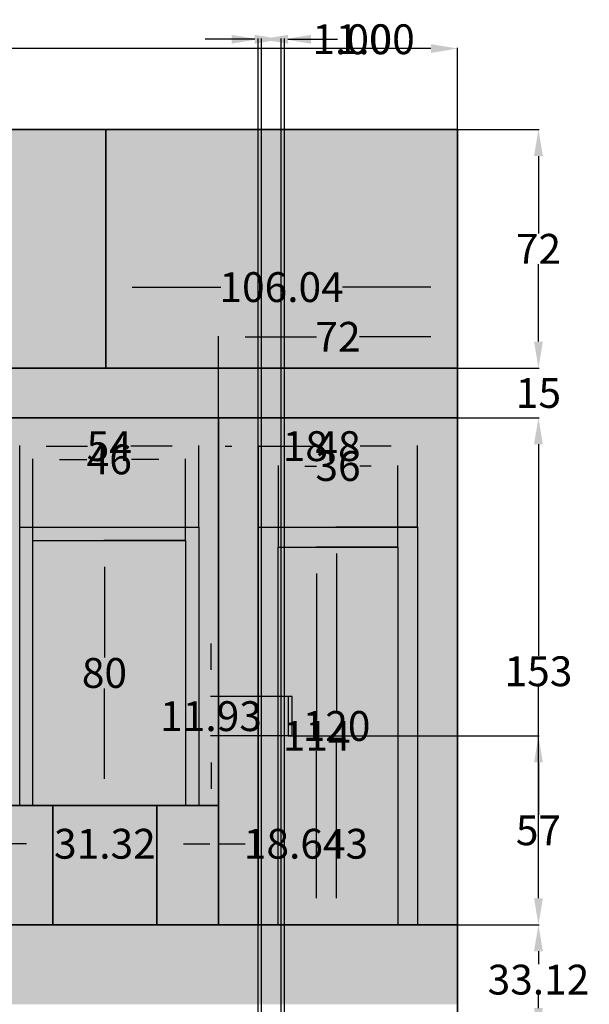
# Model space of a CAD drawing. Units: inches. Extents: x 207 to 609, y 30 to 576.
# Tile 4 of 4: x 418 to 589, y 279 to 576. Entities that reach past the tile are written whole.
import ezdxf

# ---------------------------------------------------------------- set-up
doc = ezdxf.new("R2010")
doc.units = ezdxf.units.IN
doc.header["$MEASUREMENT"] = 0
for name, color, linetype, lineweight in [('A-ANNO-DIMS', 2, 'Continuous', 18), ('A-DOOR', 3, 'Continuous', 25), ('A-ELEV', 7, 'Continuous', 35), ('A-ELEV-PATT', 251, 'Continuous', 13), ('A-ELEV-PATT-WOOD', 19, 'Continuous', 13), ('A-GLAZ', 4, 'Continuous', 25), ('A-GLAZ-PATT', 49, 'Continuous', 13)]:
    doc.layers.add(name, color=color, linetype=linetype, lineweight=lineweight)
doc.styles.get("Standard").update_dxf_attribs({"font": 'arial.ttf'})
doc.dimstyles.get("Standard").update_dxf_attribs({"dimtxt": 9, "dimasz": 8, "dimexe": 0.18, "dimexo": 0.0625, "dimgap": 0.09, "dimtad": 0, "dimtih": 1, "dimtoh": 1, "dimdec": 0, "dimzin": 0, "dimdsep": 46, "dimlunit": 3, "dimtxsty": 'Standard', "dimcen": 0.09, "dimadec": 0, "dimazin": 0, "dimtfac": 1, "dimtdec": 0, "dimtofl": 0, "dimtmove": 0, "dimatfit": 3, "dimfxl": 1, "dimtolj": 1, "dimtzin": 0, "dimarcsym": 0})

# ---------------------------------------------------------------- blocks, each defined once
blk = doc.blocks.new('*D7')
at = {"layer": 'A-ANNO-DIMS', "color": 0, "lineweight": -2, "transparency": 16777216}
for p, q in [((249.7, 542.85), (249.7, 567.42)), ((257.7, 567.24), (389.68, 567.24)), ((541.7, 567.24), (409.71, 567.24)), ((549.7, 542.85), (549.7, 567.42))]:
    blk.add_line(p, q, dxfattribs=at)
at = {"layer": 'A-ANNO-DIMS', "color": 0, "transparency": 16777216}
for points in [[(257.7, 568.57), (257.7, 565.9), (249.7, 567.24)], [(541.7, 568.57), (541.7, 565.9), (549.7, 567.24)]]:
    blk.add_solid(points, dxfattribs=at)
at = {"layer": 'Defpoints', "color": 0, "transparency": 16777216}
for p in [(549.7, 567.24), (249.7, 542.79), (549.7, 542.79)]:
    blk.add_point(p, dxfattribs=at)
at = {"layer": 'A-ANNO-DIMS', "color": 0, "transparency": 16777216, "insert": (399.7, 567.24), "char_height": 9, "attachment_point": 5}
blk.add_mtext('\\A1;300', dxfattribs=at)
blk = doc.blocks.new('*D9')
at = {"layer": 'A-ANNO-DIMS', "color": 0, "lineweight": -2, "transparency": 16777216}
for p, q in [((443.66, 470.85), (443.66, 495.42)), ((451.66, 495.24), (478.35, 495.24)), ((541.7, 495.24), (515.01, 495.24)), ((549.7, 470.85), (549.7, 495.42))]:
    blk.add_line(p, q, dxfattribs=at)
at = {"layer": 'A-ANNO-DIMS', "color": 0, "transparency": 16777216}
for points in [[(451.66, 496.57), (451.66, 493.9), (443.66, 495.24)], [(541.7, 496.57), (541.7, 493.9), (549.7, 495.24)]]:
    blk.add_solid(points, dxfattribs=at)
at = {"layer": 'Defpoints', "color": 0, "transparency": 16777216}
for p in [(549.7, 495.24), (443.66, 470.79), (549.7, 470.79)]:
    blk.add_point(p, dxfattribs=at)
at = {"layer": 'A-ANNO-DIMS', "color": 0, "transparency": 16777216, "insert": (496.68, 495.24), "char_height": 9, "attachment_point": 5}
blk.add_mtext('\\A1;106.04', dxfattribs=at)
blk = doc.blocks.new('*D22')
at = {"layer": 'A-ANNO-DIMS', "color": 0, "lineweight": -2, "transparency": 16777216}
for p, q in [((549.76, 302.79), (574.33, 302.79)), ((574.15, 294.79), (574.15, 290.91)), ((574.15, 277.66), (574.15, 281.54)), ((534.66, 269.66), (574.33, 269.66))]:
    blk.add_line(p, q, dxfattribs=at)
at = {"layer": 'A-ANNO-DIMS', "color": 0, "transparency": 16777216}
for points in [[(572.81, 294.79), (575.48, 294.79), (574.15, 302.79)], [(572.81, 277.66), (575.48, 277.66), (574.15, 269.66)]]:
    blk.add_solid(points, dxfattribs=at)
at = {"layer": 'Defpoints', "color": 0, "transparency": 16777216}
for p in [(549.7, 302.79), (574.15, 302.79), (534.6, 269.66)]:
    blk.add_point(p, dxfattribs=at)
at = {"layer": 'A-ANNO-DIMS', "color": 0, "transparency": 16777216, "insert": (574.15, 286.23), "char_height": 9, "attachment_point": 5}
blk.add_mtext('\\A1;33.12', dxfattribs=at)
blk = doc.blocks.new('*D23')
at = {"layer": 'A-ANNO-DIMS', "color": 0, "lineweight": -2, "transparency": 16777216}
for p, q in [((549.76, 455.79), (574.33, 455.79)), ((574.15, 447.79), (574.15, 383.97)), ((574.15, 310.79), (574.15, 374.6)), ((549.76, 302.79), (574.33, 302.79))]:
    blk.add_line(p, q, dxfattribs=at)
at = {"layer": 'A-ANNO-DIMS', "color": 0, "transparency": 16777216}
for points in [[(572.81, 447.79), (575.48, 447.79), (574.15, 455.79)], [(572.81, 310.79), (575.48, 310.79), (574.15, 302.79)]]:
    blk.add_solid(points, dxfattribs=at)
at = {"layer": 'Defpoints', "color": 0, "transparency": 16777216}
for p in [(549.7, 455.79), (574.15, 455.79), (549.7, 302.79)]:
    blk.add_point(p, dxfattribs=at)
at = {"layer": 'A-ANNO-DIMS', "color": 0, "transparency": 16777216, "insert": (574.15, 379.29), "char_height": 9, "attachment_point": 5}
blk.add_mtext('\\A1;153', dxfattribs=at)
blk = doc.blocks.new('*D24')
at = {"layer": 'A-ANNO-DIMS', "color": 0, "lineweight": -2, "transparency": 16777216}
for p, q in [((574.15, 478.79), (574.15, 486.79)), ((549.76, 470.79), (574.33, 470.79)), ((549.76, 455.79), (574.33, 455.79)), ((574.15, 447.79), (574.15, 439.79))]:
    blk.add_line(p, q, dxfattribs=at)
at = {"layer": 'A-ANNO-DIMS', "color": 0, "transparency": 16777216}
for points in [[(572.81, 478.79), (575.48, 478.79), (574.15, 470.79)], [(572.81, 447.79), (575.48, 447.79), (574.15, 455.79)]]:
    blk.add_solid(points, dxfattribs=at)
at = {"layer": 'Defpoints', "color": 0, "transparency": 16777216}
for p in [(549.7, 470.79), (574.15, 470.79), (549.7, 455.79)]:
    blk.add_point(p, dxfattribs=at)
at = {"layer": 'A-ANNO-DIMS', "color": 0, "transparency": 16777216, "insert": (574.15, 463.29), "char_height": 9, "attachment_point": 5}
blk.add_mtext('\\A1;15', dxfattribs=at)
blk = doc.blocks.new('*D25')
at = {"layer": 'A-ANNO-DIMS', "color": 0, "lineweight": -2, "transparency": 16777216}
for p, q in [((549.76, 542.79), (574.33, 542.79)), ((574.15, 534.79), (574.15, 511.39)), ((574.15, 478.79), (574.15, 502.18)), ((549.76, 470.79), (574.33, 470.79))]:
    blk.add_line(p, q, dxfattribs=at)
at = {"layer": 'A-ANNO-DIMS', "color": 0, "transparency": 16777216}
for points in [[(572.81, 534.79), (575.48, 534.79), (574.15, 542.79)], [(572.81, 478.79), (575.48, 478.79), (574.15, 470.79)]]:
    blk.add_solid(points, dxfattribs=at)
at = {"layer": 'Defpoints', "color": 0, "transparency": 16777216}
for p in [(549.7, 542.79), (574.15, 542.79), (549.7, 470.79)]:
    blk.add_point(p, dxfattribs=at)
at = {"layer": 'A-ANNO-DIMS', "color": 0, "transparency": 16777216, "insert": (574.15, 506.79), "char_height": 9, "attachment_point": 5}
blk.add_mtext('\\A1;72', dxfattribs=at)
blk = doc.blocks.new('*D42')
at = {"layer": 'A-ANNO-DIMS', "color": 0, "lineweight": -2, "transparency": 16777216}
for p, q in [((477.7, 455.85), (477.7, 480.42)), ((485.7, 480.24), (507.24, 480.24)), ((541.7, 480.24), (520.15, 480.24)), ((549.7, 455.85), (549.7, 480.42))]:
    blk.add_line(p, q, dxfattribs=at)
at = {"layer": 'A-ANNO-DIMS', "color": 0, "transparency": 16777216}
for points in [[(485.7, 481.57), (485.7, 478.9), (477.7, 480.24)], [(541.7, 481.57), (541.7, 478.9), (549.7, 480.24)]]:
    blk.add_solid(points, dxfattribs=at)
at = {"layer": 'Defpoints', "color": 0, "transparency": 16777216}
for p in [(549.7, 480.24), (477.7, 455.79), (549.7, 455.79)]:
    blk.add_point(p, dxfattribs=at)
at = {"layer": 'A-ANNO-DIMS', "color": 0, "transparency": 16777216, "insert": (513.7, 480.24), "char_height": 9, "attachment_point": 5}
blk.add_mtext('\\A1;72', dxfattribs=at)
blk = doc.blocks.new('*D44')
at = {"layer": 'A-ANNO-DIMS', "color": 0, "lineweight": -2, "transparency": 16777216}
for p, q in [((417.7, 422.85), (417.7, 447.42)), ((425.7, 447.24), (438.18, 447.24)), ((463.7, 447.24), (451.21, 447.24)), ((471.7, 422.85), (471.7, 447.42))]:
    blk.add_line(p, q, dxfattribs=at)
at = {"layer": 'A-ANNO-DIMS', "color": 0, "transparency": 16777216}
for points in [[(425.7, 448.57), (425.7, 445.9), (417.7, 447.24)], [(463.7, 448.57), (463.7, 445.9), (471.7, 447.24)]]:
    blk.add_solid(points, dxfattribs=at)
at = {"layer": 'Defpoints', "color": 0, "transparency": 16777216}
for p in [(471.7, 447.24), (417.7, 422.79), (471.7, 422.79)]:
    blk.add_point(p, dxfattribs=at)
at = {"layer": 'A-ANNO-DIMS', "color": 0, "transparency": 16777216, "insert": (444.7, 447.24), "char_height": 9, "attachment_point": 5}
blk.add_mtext('\\A1;54', dxfattribs=at)
blk = doc.blocks.new('*D45')
at = {"layer": 'A-ANNO-DIMS', "color": 0, "lineweight": -2, "transparency": 16777216}
for p, q in [((471.7, 422.85), (471.7, 447.42)), ((479.7, 447.24), (481.7, 447.24)), ((489.7, 422.85), (489.7, 447.42)), ((489.7, 447.24), (497.7, 447.24))]:
    blk.add_line(p, q, dxfattribs=at)
at = {"layer": 'A-ANNO-DIMS', "color": 0, "transparency": 16777216}
for points in [[(479.7, 448.57), (479.7, 445.9), (471.7, 447.24)], [(481.7, 448.57), (481.7, 445.9), (489.7, 447.24)]]:
    blk.add_solid(points, dxfattribs=at)
at = {"layer": 'Defpoints', "color": 0, "transparency": 16777216}
for p in [(489.7, 447.24), (471.7, 422.79), (489.7, 422.79)]:
    blk.add_point(p, dxfattribs=at)
at = {"layer": 'A-ANNO-DIMS', "color": 0, "transparency": 16777216, "insert": (503.82, 447.24), "char_height": 9, "attachment_point": 5}
blk.add_mtext('\\A1;18', dxfattribs=at)
blk = doc.blocks.new('*D46')
at = {"layer": 'A-ANNO-DIMS', "color": 0, "lineweight": -2, "transparency": 16777216}
for p, q in [((489.7, 422.85), (489.7, 447.42)), ((497.7, 447.24), (506.97, 447.24)), ((529.7, 447.24), (520.42, 447.24)), ((537.7, 422.85), (537.7, 447.42))]:
    blk.add_line(p, q, dxfattribs=at)
at = {"layer": 'A-ANNO-DIMS', "color": 0, "transparency": 16777216}
for points in [[(497.7, 448.57), (497.7, 445.9), (489.7, 447.24)], [(529.7, 448.57), (529.7, 445.9), (537.7, 447.24)]]:
    blk.add_solid(points, dxfattribs=at)
at = {"layer": 'Defpoints', "color": 0, "transparency": 16777216}
for p in [(537.7, 447.24), (489.7, 422.79), (537.7, 422.79)]:
    blk.add_point(p, dxfattribs=at)
at = {"layer": 'A-ANNO-DIMS', "color": 0, "transparency": 16777216, "insert": (513.7, 447.24), "char_height": 9, "attachment_point": 5}
blk.add_mtext('\\A1;48', dxfattribs=at)
blk = doc.blocks.new('*D48')
at = {"layer": 'A-ANNO-DIMS', "color": 0, "lineweight": -2, "transparency": 16777216}
for p, q in [((367.66, 302.85), (367.66, 327.42)), ((375.66, 327.24), (382.4, 327.24)), ((419.73, 327.24), (413, 327.24)), ((427.73, 302.85), (427.73, 327.42))]:
    blk.add_line(p, q, dxfattribs=at)
at = {"layer": 'A-ANNO-DIMS', "color": 0, "transparency": 16777216}
for points in [[(375.66, 328.57), (375.66, 325.9), (367.66, 327.24)], [(419.73, 328.57), (419.73, 325.9), (427.73, 327.24)]]:
    blk.add_solid(points, dxfattribs=at)
at = {"layer": 'Defpoints', "color": 0, "transparency": 16777216}
for p in [(427.73, 327.24), (367.66, 302.79), (427.73, 302.79)]:
    blk.add_point(p, dxfattribs=at)
at = {"layer": 'A-ANNO-DIMS', "color": 0, "transparency": 16777216, "insert": (397.7, 327.24), "char_height": 9, "attachment_point": 5}
blk.add_mtext('\\A1;60.07', dxfattribs=at)
blk = doc.blocks.new('*D49')
at = {"layer": 'A-ANNO-DIMS', "color": 0, "lineweight": -2, "transparency": 16777216}
for p, q in [((419.73, 327.24), (411.73, 327.24)), ((427.73, 302.85), (427.73, 327.42)), ((459.05, 302.85), (459.05, 327.42)), ((467.05, 327.24), (475.05, 327.24))]:
    blk.add_line(p, q, dxfattribs=at)
at = {"layer": 'A-ANNO-DIMS', "color": 0, "transparency": 16777216}
for points in [[(419.73, 328.57), (419.73, 325.9), (427.73, 327.24)], [(467.05, 328.57), (467.05, 325.9), (459.05, 327.24)]]:
    blk.add_solid(points, dxfattribs=at)
at = {"layer": 'Defpoints', "color": 0, "transparency": 16777216}
for p in [(459.05, 327.24), (427.73, 302.79), (459.05, 302.79)]:
    blk.add_point(p, dxfattribs=at)
at = {"layer": 'A-ANNO-DIMS', "color": 0, "transparency": 16777216, "insert": (443.39, 327.24), "char_height": 9, "attachment_point": 5}
blk.add_mtext('\\A1;31.32', dxfattribs=at)
blk = doc.blocks.new('*D50')
at = {"layer": 'A-ANNO-DIMS', "color": 0, "lineweight": -2, "transparency": 16777216}
for p, q in [((459.05, 302.85), (459.05, 327.42)), ((467.05, 327.24), (469.7, 327.24)), ((477.7, 302.85), (477.7, 327.42)), ((477.7, 327.24), (485.7, 327.24))]:
    blk.add_line(p, q, dxfattribs=at)
at = {"layer": 'A-ANNO-DIMS', "color": 0, "transparency": 16777216}
for points in [[(467.05, 328.57), (467.05, 325.9), (459.05, 327.24)], [(469.7, 328.57), (469.7, 325.9), (477.7, 327.24)]]:
    blk.add_solid(points, dxfattribs=at)
at = {"layer": 'Defpoints', "color": 0, "transparency": 16777216}
for p in [(477.7, 327.24), (459.05, 302.79), (477.7, 302.79)]:
    blk.add_point(p, dxfattribs=at)
at = {"layer": 'A-ANNO-DIMS', "color": 0, "transparency": 16777216, "insert": (504.04, 327.24), "char_height": 9, "attachment_point": 5}
blk.add_mtext('\\A1;18.643', dxfattribs=at)
blk = doc.blocks.new('*D53')
at = {"layer": 'A-ANNO-DIMS', "color": 0, "lineweight": -2, "transparency": 16777216}
for p, q in [((421.7, 418.85), (421.7, 443.42)), ((429.7, 443.24), (437.98, 443.24)), ((459.7, 443.24), (451.41, 443.24)), ((467.7, 418.85), (467.7, 443.42))]:
    blk.add_line(p, q, dxfattribs=at)
at = {"layer": 'A-ANNO-DIMS', "color": 0, "transparency": 16777216}
for points in [[(429.7, 444.57), (429.7, 441.9), (421.7, 443.24)], [(459.7, 444.57), (459.7, 441.9), (467.7, 443.24)]]:
    blk.add_solid(points, dxfattribs=at)
at = {"layer": 'Defpoints', "color": 0, "transparency": 16777216}
for p in [(467.7, 443.24), (421.7, 418.79), (467.7, 418.79)]:
    blk.add_point(p, dxfattribs=at)
at = {"layer": 'A-ANNO-DIMS', "color": 0, "transparency": 16777216, "insert": (444.7, 443.24), "char_height": 9, "attachment_point": 5}
blk.add_mtext('\\A1;46', dxfattribs=at)
blk = doc.blocks.new('*D54')
at = {"layer": 'A-ANNO-DIMS', "color": 0, "lineweight": -2, "transparency": 16777216}
for p, q in [((467.63, 418.79), (443.07, 418.79)), ((443.25, 410.79), (443.25, 383.47)), ((443.25, 346.79), (443.25, 374.1)), ((467.63, 338.79), (443.07, 338.79))]:
    blk.add_line(p, q, dxfattribs=at)
at = {"layer": 'A-ANNO-DIMS', "color": 0, "transparency": 16777216}
for points in [[(441.91, 410.79), (444.58, 410.79), (443.25, 418.79)], [(441.91, 346.79), (444.58, 346.79), (443.25, 338.79)]]:
    blk.add_solid(points, dxfattribs=at)
at = {"layer": 'Defpoints', "color": 0, "transparency": 16777216}
for p in [(443.25, 418.79), (467.7, 418.79), (467.7, 338.79)]:
    blk.add_point(p, dxfattribs=at)
at = {"layer": 'A-ANNO-DIMS', "color": 0, "transparency": 16777216, "insert": (443.25, 378.79), "char_height": 9, "attachment_point": 5}
blk.add_mtext('\\A1;80', dxfattribs=at)
blk = doc.blocks.new('*D55')
at = {"layer": 'A-ANNO-DIMS', "color": 0, "lineweight": -2, "transparency": 16777216}
for p, q in [((537.63, 422.79), (513.07, 422.79)), ((513.25, 414.79), (513.25, 367.47)), ((513.25, 310.79), (513.25, 358.1)), ((537.63, 302.79), (513.07, 302.79))]:
    blk.add_line(p, q, dxfattribs=at)
at = {"layer": 'A-ANNO-DIMS', "color": 0, "transparency": 16777216}
for points in [[(511.91, 414.79), (514.58, 414.79), (513.25, 422.79)], [(511.91, 310.79), (514.58, 310.79), (513.25, 302.79)]]:
    blk.add_solid(points, dxfattribs=at)
at = {"layer": 'Defpoints', "color": 0, "transparency": 16777216}
for p in [(513.25, 422.79), (537.7, 422.79), (537.7, 302.79)]:
    blk.add_point(p, dxfattribs=at)
at = {"layer": 'A-ANNO-DIMS', "color": 0, "transparency": 16777216, "insert": (513.25, 362.79), "char_height": 9, "attachment_point": 5}
blk.add_mtext('\\A1;120', dxfattribs=at)
blk = doc.blocks.new('*D56')
at = {"layer": 'A-ANNO-DIMS', "color": 0, "lineweight": -2, "transparency": 16777216}
for p, q in [((495.7, 416.85), (495.7, 441.42)), ((503.7, 441.24), (507.17, 441.24)), ((523.7, 441.24), (520.23, 441.24)), ((531.7, 416.85), (531.7, 441.42))]:
    blk.add_line(p, q, dxfattribs=at)
at = {"layer": 'A-ANNO-DIMS', "color": 0, "transparency": 16777216}
for points in [[(503.7, 442.57), (503.7, 439.9), (495.7, 441.24)], [(523.7, 442.57), (523.7, 439.9), (531.7, 441.24)]]:
    blk.add_solid(points, dxfattribs=at)
at = {"layer": 'Defpoints', "color": 0, "transparency": 16777216}
for p in [(531.7, 441.24), (495.7, 416.79), (531.7, 416.79)]:
    blk.add_point(p, dxfattribs=at)
at = {"layer": 'A-ANNO-DIMS', "color": 0, "transparency": 16777216, "insert": (513.7, 441.24), "char_height": 9, "attachment_point": 5}
blk.add_mtext('\\A1;36', dxfattribs=at)
blk = doc.blocks.new('*D57')
at = {"layer": 'A-ANNO-DIMS', "color": 0, "lineweight": -2, "transparency": 16777216}
for p, q in [((531.63, 416.79), (507.07, 416.79)), ((507.25, 408.79), (507.25, 364.39)), ((507.25, 310.79), (507.25, 355.18)), ((531.63, 302.79), (507.07, 302.79))]:
    blk.add_line(p, q, dxfattribs=at)
at = {"layer": 'A-ANNO-DIMS', "color": 0, "transparency": 16777216}
for points in [[(505.91, 408.79), (508.58, 408.79), (507.25, 416.79)], [(505.91, 310.79), (508.58, 310.79), (507.25, 302.79)]]:
    blk.add_solid(points, dxfattribs=at)
at = {"layer": 'Defpoints', "color": 0, "transparency": 16777216}
for p in [(507.25, 416.79), (531.7, 416.79), (531.7, 302.79)]:
    blk.add_point(p, dxfattribs=at)
at = {"layer": 'A-ANNO-DIMS', "color": 0, "transparency": 16777216, "insert": (507.25, 359.79), "char_height": 9, "attachment_point": 5}
blk.add_mtext('\\A1;114', dxfattribs=at)
blk = doc.blocks.new('*D58')
at = {"layer": 'A-ANNO-DIMS', "color": 0, "lineweight": -2, "transparency": 16777216}
for p, q in [((499.91, 359.79), (574.33, 359.79)), ((574.15, 351.79), (574.15, 335.95)), ((574.15, 310.79), (574.15, 326.62)), ((531.76, 302.79), (574.33, 302.79))]:
    blk.add_line(p, q, dxfattribs=at)
at = {"layer": 'A-ANNO-DIMS', "color": 0, "transparency": 16777216}
for points in [[(572.81, 351.79), (575.48, 351.79), (574.15, 359.79)], [(572.81, 310.79), (575.48, 310.79), (574.15, 302.79)]]:
    blk.add_solid(points, dxfattribs=at)
at = {"layer": 'Defpoints', "color": 0, "transparency": 16777216}
for p in [(499.85, 359.79), (574.15, 359.79), (531.7, 302.79)]:
    blk.add_point(p, dxfattribs=at)
at = {"layer": 'A-ANNO-DIMS', "color": 0, "transparency": 16777216, "insert": (574.15, 331.29), "char_height": 9, "attachment_point": 5}
blk.add_mtext('\\A1;57', dxfattribs=at)
blk = doc.blocks.new('*D59')
at = {"layer": 'A-ANNO-DIMS', "color": 0, "lineweight": -2, "transparency": 16777216}
for p, q in [((475.4, 379.72), (475.4, 387.72)), ((499.79, 371.72), (475.22, 371.72)), ((499.79, 359.79), (475.22, 359.79)), ((475.4, 351.79), (475.4, 343.79))]:
    blk.add_line(p, q, dxfattribs=at)
at = {"layer": 'A-ANNO-DIMS', "color": 0, "transparency": 16777216}
for points in [[(474.07, 379.72), (476.74, 379.72), (475.4, 371.72)], [(474.07, 351.79), (476.74, 351.79), (475.4, 359.79)]]:
    blk.add_solid(points, dxfattribs=at)
at = {"layer": 'Defpoints', "color": 0, "transparency": 16777216}
for p in [(475.4, 371.72), (499.85, 371.72), (499.85, 359.79)]:
    blk.add_point(p, dxfattribs=at)
at = {"layer": 'A-ANNO-DIMS', "color": 0, "transparency": 16777216, "insert": (475.4, 365.75), "char_height": 9, "attachment_point": 5}
blk.add_mtext('\\A1;11.93', dxfattribs=at)
blk = doc.blocks.new('*D81')
at = {"layer": 'A-ANNO-DIMS', "color": 0, "lineweight": -2, "transparency": 16777216}
for p, q in [((481.58, 570.04), (473.58, 570.04)), ((489.58, 151.35), (489.58, 570.22)), ((490.58, 151.35), (490.58, 570.22)), ((498.58, 570.04), (506.58, 570.04))]:
    blk.add_line(p, q, dxfattribs=at)
at = {"layer": 'A-ANNO-DIMS', "color": 0, "transparency": 16777216}
for points in [[(481.58, 571.37), (481.58, 568.7), (489.58, 570.04)], [(498.58, 571.37), (498.58, 568.7), (490.58, 570.04)]]:
    blk.add_solid(points, dxfattribs=at)
at = {"layer": 'Defpoints', "color": 0, "transparency": 16777216}
for p in [(490.58, 570.04), (489.58, 151.29), (490.58, 151.29)]:
    blk.add_point(p, dxfattribs=at)
at = {"layer": 'A-ANNO-DIMS', "color": 0, "transparency": 16777216, "insert": (517.92, 570.04), "char_height": 9, "attachment_point": 5}
blk.add_mtext('\\A1;1.00', dxfattribs=at)
blk = doc.blocks.new('*D82')
at = {"layer": 'A-ANNO-DIMS', "color": 0, "lineweight": -2, "transparency": 16777216}
for p, q in [((488.58, 570.04), (480.58, 570.04)), ((496.58, 151.35), (496.58, 570.22)), ((497.58, 151.35), (497.58, 570.22)), ((505.58, 570.04), (513.58, 570.04))]:
    blk.add_line(p, q, dxfattribs=at)
at = {"layer": 'A-ANNO-DIMS', "color": 0, "transparency": 16777216}
for points in [[(488.58, 571.37), (488.58, 568.7), (496.58, 570.04)], [(505.58, 571.37), (505.58, 568.7), (497.58, 570.04)]]:
    blk.add_solid(points, dxfattribs=at)
at = {"layer": 'Defpoints', "color": 0, "transparency": 16777216}
for p in [(497.58, 570.04), (496.58, 151.29), (497.58, 151.29)]:
    blk.add_point(p, dxfattribs=at)
at = {"layer": 'A-ANNO-DIMS', "color": 0, "transparency": 16777216, "insert": (524.92, 570.04), "char_height": 9, "attachment_point": 5}
blk.add_mtext('\\A1;1.00', dxfattribs=at)

msp = doc.modelspace()

# ---------------------------------------------------------------- hatches: boundary and pattern name
at = {"layer": 'A-ELEV-PATT'}
h = msp.add_hatch(color=256, dxfattribs=at)
h.dxf.hatch_style = 1
h.paths.add_polyline_path([(443.656, 542.7864), (249.6956, 542.7864), (249.6956, 302.7864), (309.6956, 302.7864), (309.6956, 470.7864), (443.656, 470.7864)])
h = msp.add_hatch(color=256, dxfattribs=at)
h.dxf.hatch_style = 1
h.paths.add_polyline_path([(549.6956, 542.7864), (443.656, 542.7864), (443.656, 470.7864), (549.6956, 470.7864)])
h.paths.add_polyline_path([(549.6956, 230.7864), (249.6956, 230.7864), (249.6956, 218.7864), (549.6956, 218.7864)])
h.paths.add_polyline_path([(377.5808, 80.7864), (265.6956, 80.7864), (265.6956, 62.7864), (377.5808, 62.7864)])
h.paths.add_polyline_path([(549.6956, 71.7864), (443.5808, 71.7864), (443.5808, 62.7864), (549.6956, 62.7864)])
h = msp.add_hatch(color=256, dxfattribs=at)
h.dxf.hatch_style = 1
h.paths.add_polyline_path([(549.6956, 470.7864), (309.6956, 470.7864), (309.6956, 278.7864), (549.6956, 278.7864), (549.6956, 302.7864), (324.6956, 302.7864), (324.6956, 455.7864), (549.6956, 455.7864)])
h = msp.add_hatch(color=256, dxfattribs=at)
h.dxf.hatch_style = 1
h.paths.add_polyline_path([(477.6956, 455.7864), (411.6956, 455.7864), (411.6956, 338.7864), (417.6956, 338.7864), (417.6956, 422.7864), (471.6956, 422.7864), (471.6956, 338.7864), (477.6956, 338.7864)])
at = {"layer": 'A-ELEV-PATT', "transparency": 33554656}
h = msp.add_hatch(color=256, dxfattribs=at)
h.set_gradient(color1=(215, 235, 210), color2=(32, 70, 27), name='INVCURVED')
h.paths.add_polyline_path([(537.6956, 422.7864), (537.6956, 338.7864), (549.6956, 338.7864), (549.6956, 455.7864), (477.6956, 455.7864), (477.6956, 338.7864), (489.6956, 338.7864), (489.6956, 422.7864)])
h = msp.add_hatch(color=256, dxfattribs=at)
h.paths.add_polyline_path([(367.6635, 338.7864), (324.6956, 338.7864), (324.6956, 302.7864), (367.6635, 302.7864)])
h.paths.add_polyline_path([(427.7296, 338.7864), (367.6635, 338.7864), (367.6635, 302.7864), (427.7296, 302.7864)])
h.paths.add_polyline_path([(459.0525, 338.7864), (427.7296, 338.7864), (427.7296, 302.7864), (459.0525, 302.7864)])
h.paths.add_polyline_path([(477.6956, 338.7864), (459.0525, 338.7864), (459.0525, 302.7864), (477.6956, 302.7864)])
at = {"layer": 'A-ELEV-PATT-WOOD', "transparency": 33554656}
for points in [[(471.6956, 422.7864), (417.6956, 422.7864), (417.6956, 338.7864), (421.6956, 338.7864), (421.6956, 418.7864), (467.6956, 418.7864), (467.6956, 338.7864), (471.6956, 338.7864)], [(537.6956, 422.7864), (489.6956, 422.7864), (489.6956, 338.7864), (495.6956, 338.7864), (495.6956, 416.7864), (531.6956, 416.7864), (531.6956, 338.7864), (537.6956, 338.7864)], [(537.6956, 422.7864), (489.6956, 422.7864), (489.6956, 338.7864), (495.6956, 338.7864), (495.6956, 416.7864), (531.6956, 416.7864), (531.6956, 338.7864), (537.6956, 338.7864)]]:
    msp.add_hatch(color=256, dxfattribs=at).paths.add_polyline_path(points)
h = msp.add_hatch(color=256, dxfattribs=at)
h.paths.add_polyline_path([(490.5808, 151.2864), (489.5808, 151.2864), (489.5808, 139.2864), (490.5808, 139.2864)])
h.paths.add_polyline_path([(497.5808, 151.2864), (496.5808, 151.2864), (496.5808, 139.2864), (497.5808, 139.2864)])
h.paths.add_polyline_path([(499.8522, 371.716), (498.6956, 371.716), (498.6956, 359.7864), (499.8522, 359.7864)])
h = msp.add_hatch(color=256, dxfattribs=at)
h.paths.add_polyline_path([(495.6956, 338.7864), (489.6956, 338.7864), (489.6956, 302.7864), (495.6956, 302.7864)])
h.paths.add_polyline_path([(537.6956, 338.7864), (531.6956, 338.7864), (531.6956, 302.7864), (537.6956, 302.7864)])
at = {"layer": 'A-GLAZ-PATT', "transparency": 33554656}
for points in [[(467.6956, 418.7864), (421.6956, 418.7864), (421.6956, 338.7864), (467.6956, 338.7864)], [(531.6956, 338.7864), (495.6956, 338.7864), (495.6956, 302.7864), (531.6956, 302.7864)]]:
    msp.add_hatch(color=256, dxfattribs=at).paths.add_polyline_path(points)
h = msp.add_hatch(color=256, dxfattribs=at)
h.paths.add_polyline_path([(531.6956, 416.7864), (495.6956, 416.7864), (495.6956, 338.7864), (531.6956, 338.7864)])
h.paths.add_polyline_path([(499.8522, 359.7864), (498.6956, 359.7864), (498.6956, 371.716), (499.8522, 371.716)], flags=16)
h = msp.add_hatch(color=256, dxfattribs=at)
h.paths.add_polyline_path([(489.6956, 338.7864), (477.6956, 338.7864), (477.6956, 302.7864), (489.6956, 302.7864)])
h.paths.add_polyline_path([(549.6956, 338.7864), (537.6956, 338.7864), (537.6956, 302.7864), (549.6956, 302.7864)])

# ---------------------------------------------------------------- linework, layer by layer
at = {"layer": 'A-DOOR'}
for p, q in [((499.8522, 371.716), (498.6956, 371.716)), ((498.6956, 371.716), (498.6956, 359.7864)), ((499.8522, 359.7864), (499.8522, 371.716)), ((498.6956, 359.7864), (499.8522, 359.7864))]:
    msp.add_line(p, q, dxfattribs=at)
for points in [[(489.6956, 302.7864), (489.6956, 422.7864), (537.6956, 422.7864), (537.6956, 302.7864)], [(495.6956, 302.7864), (495.6956, 416.7864), (531.6956, 416.7864), (531.6956, 302.7864)]]:
    msp.add_lwpolyline(points, dxfattribs=at)
at = {"layer": 'A-ELEV'}
for p, q in [((249.6956, 542.7864), (549.6956, 542.7864)), ((443.656, 470.7864), (443.656, 542.7864)), ((549.6956, 542.7864), (549.6956, 62.7864)), ((309.6956, 470.7864), (549.6956, 470.7864)), ((324.6956, 455.7864), (549.6956, 455.7864)), ((477.6956, 455.7864), (477.6956, 302.7864)), ((477.6956, 338.7864), (324.6956, 338.7864)), ((427.7296, 338.7864), (427.7296, 302.7864)), ((459.0525, 338.7864), (459.0525, 302.7864)), ((549.6956, 302.7864), (324.6956, 302.7864))]:
    msp.add_line(p, q, dxfattribs=at)
at = {"layer": 'A-GLAZ'}
for points in [[(417.6956, 338.7864), (417.6956, 422.7864), (471.6956, 422.7864), (471.6956, 338.7864)], [(421.6956, 338.7864), (421.6956, 418.7864), (467.6956, 418.7864), (467.6956, 338.7864)]]:
    msp.add_lwpolyline(points, dxfattribs=at)

# ---------------------------------------------------------------- dimensions: what is measured, and where the dimension line sits
at = {"layer": 'A-ANNO-DIMS'}
for base, p1, p2, override, picture, middle in [((490.5808, 570.0364), (489.5808, 151.2864), (490.5808, 151.2864), {"dimdec": 2, "dimlfac": 1, "dimrnd": 0, "dimzin": 0, "dimdsep": 46, "dimlunit": 2}, '*D81', (517.9208, 570.0364)), ((497.5808, 570.0364), (496.5808, 151.2864), (497.5808, 151.2864), {"dimdec": 2, "dimlfac": 1, "dimrnd": 0, "dimzin": 0, "dimdsep": 46, "dimlunit": 2}, '*D82', (524.9208, 570.0364)), ((549.6956, 567.2364), (249.6956, 542.7864), (549.6956, 542.7864), {"dimdec": 0, "dimlfac": 1, "dimrnd": 0, "dimzin": 0, "dimdsep": 46, "dimlunit": 2}, '*D7', (399.6956, 567.2364)), ((549.6956, 495.2364), (443.656, 470.7864), (549.6956, 470.7864), {"dimdec": 2, "dimlfac": 1, "dimrnd": 0, "dimzin": 0, "dimdsep": 46, "dimlunit": 2}, '*D9', (496.6758, 495.2364)), ((471.6956, 447.2364), (417.6956, 422.7864), (471.6956, 422.7864), {"dimdec": 0, "dimlfac": 1, "dimrnd": 0, "dimzin": 0, "dimdsep": 46, "dimlunit": 2}, '*D44', (444.6956, 447.2364)), ((489.6956, 447.2364), (471.6956, 422.7864), (489.6956, 422.7864), {"dimdec": 0, "dimlfac": 1, "dimrnd": 0, "dimzin": 0, "dimdsep": 46, "dimlunit": 2}, '*D45', (503.8173, 447.2364)), ((537.6956, 447.2364), (489.6956, 422.7864), (537.6956, 422.7864), {"dimdec": 0, "dimlfac": 1, "dimrnd": 0, "dimzin": 0, "dimdsep": 46, "dimlunit": 2}, '*D46', (513.6956, 447.2364)), ((467.6956, 443.2364), (421.6956, 418.7864), (467.6956, 418.7864), {"dimdec": 0, "dimlfac": 1, "dimrnd": 0, "dimzin": 0, "dimdsep": 46, "dimlunit": 2}, '*D53', (444.6956, 443.2364)), ((531.6956, 441.2364), (495.6956, 416.7864), (531.6956, 416.7864), {"dimdec": 0, "dimlfac": 1, "dimrnd": 0, "dimzin": 0, "dimdsep": 46, "dimlunit": 2}, '*D56', (513.6956, 441.2364)), ((427.7296, 327.2364), (367.6635, 302.7864), (427.7296, 302.7864), {"dimdec": 2, "dimlfac": 1, "dimrnd": 0, "dimzin": 0, "dimdsep": 46, "dimlunit": 2}, '*D48', (397.6965, 327.2364)), ((459.0525, 327.2364), (427.7296, 302.7864), (459.0525, 302.7864), {"dimdec": 2, "dimlfac": 1, "dimrnd": 0, "dimzin": 0, "dimdsep": 46, "dimlunit": 2}, '*D49', (443.3911, 327.2364)), ((477.6956, 327.2364), (459.0525, 302.7864), (477.6956, 302.7864), {"dimdec": 3, "dimlfac": 1, "dimrnd": 0, "dimzin": 0, "dimdsep": 46, "dimlunit": 2}, '*D50', (504.0434, 327.2364))]:
    dim = msp.add_linear_dim(base=base, p1=p1, p2=p2, dimstyle='Standard', override=override, dxfattribs=at)
    dim.commit()
    dim.dimension.update_dxf_attribs({"geometry": picture, "text_midpoint": middle})
for base, p1, p2, angle, override, picture, middle in [((574.1456, 542.7864), (549.6956, 470.7864), (549.6956, 542.7864), 90, {"dimdec": 0, "dimlfac": 1, "dimrnd": 0, "dimzin": 0, "dimdsep": 46, "dimlunit": 2}, '*D25', (574.1456, 506.7864)), ((549.6956, 480.2364), (477.6956, 455.7864), (549.6956, 455.7864), 0, {"dimdec": 0, "dimlfac": 1, "dimrnd": 0, "dimzin": 0, "dimdsep": 46, "dimlunit": 2}, '*D42', (513.6956, 480.2364)), ((574.1456, 470.7864), (549.6956, 455.7864), (549.6956, 470.7864), 90, {"dimdec": 0, "dimlfac": 1, "dimrnd": 0, "dimzin": 0, "dimdsep": 46, "dimlunit": 2}, '*D24', (574.1456, 463.2864)), ((574.1456, 455.7864), (549.6956, 302.7864), (549.6956, 455.7864), 90, {"dimdec": 0, "dimlfac": 1, "dimrnd": 0, "dimzin": 0, "dimdsep": 46, "dimlunit": 2}, '*D23', (574.1456, 379.2864)), ((513.2456, 422.7864), (537.6956, 302.7864), (537.6956, 422.7864), 90, {"dimdec": 0, "dimlfac": 1, "dimrnd": 0, "dimzin": 0, "dimdsep": 46, "dimlunit": 2}, '*D55', (513.2456, 362.7864)), ((443.2456, 418.7864), (467.6956, 338.7864), (467.6956, 418.7864), 90, {"dimdec": 0, "dimlfac": 1, "dimrnd": 0, "dimzin": 0, "dimdsep": 46, "dimlunit": 2}, '*D54', (443.2456, 378.7864)), ((507.2456, 416.7864), (531.6956, 302.7864), (531.6956, 416.7864), 90, {"dimdec": 0, "dimlfac": 1, "dimrnd": 0, "dimzin": 0, "dimdsep": 46, "dimlunit": 2}, '*D57', (507.2456, 359.7864)), ((475.4022, 371.716), (499.8522, 359.7864), (499.8522, 371.716), 90, {"dimdec": 2, "dimlfac": 1, "dimrnd": 0, "dimzin": 0, "dimdsep": 46, "dimlunit": 2}, '*D59', (475.4022, 365.7512)), ((574.1456, 359.7864), (531.6956, 302.7864), (499.8522, 359.7864), 90, {"dimdec": 0, "dimlfac": 1, "dimrnd": 0, "dimzin": 0, "dimdsep": 46, "dimlunit": 2}, '*D58', (574.1456, 331.2864)), ((574.1456, 302.7864), (534.6005, 269.6636), (549.6956, 302.7864), 90, {"dimdec": 2, "dimlfac": 1, "dimrnd": 0, "dimzin": 0, "dimdsep": 46, "dimlunit": 2}, '*D22', (574.1456, 286.225))]:
    dim = msp.add_linear_dim(base=base, p1=p1, p2=p2, angle=angle, dimstyle='Standard', override=override, dxfattribs=at)
    dim.commit()
    dim.dimension.update_dxf_attribs({"geometry": picture, "text_midpoint": middle})

doc.saveas('drawing.dxf')
